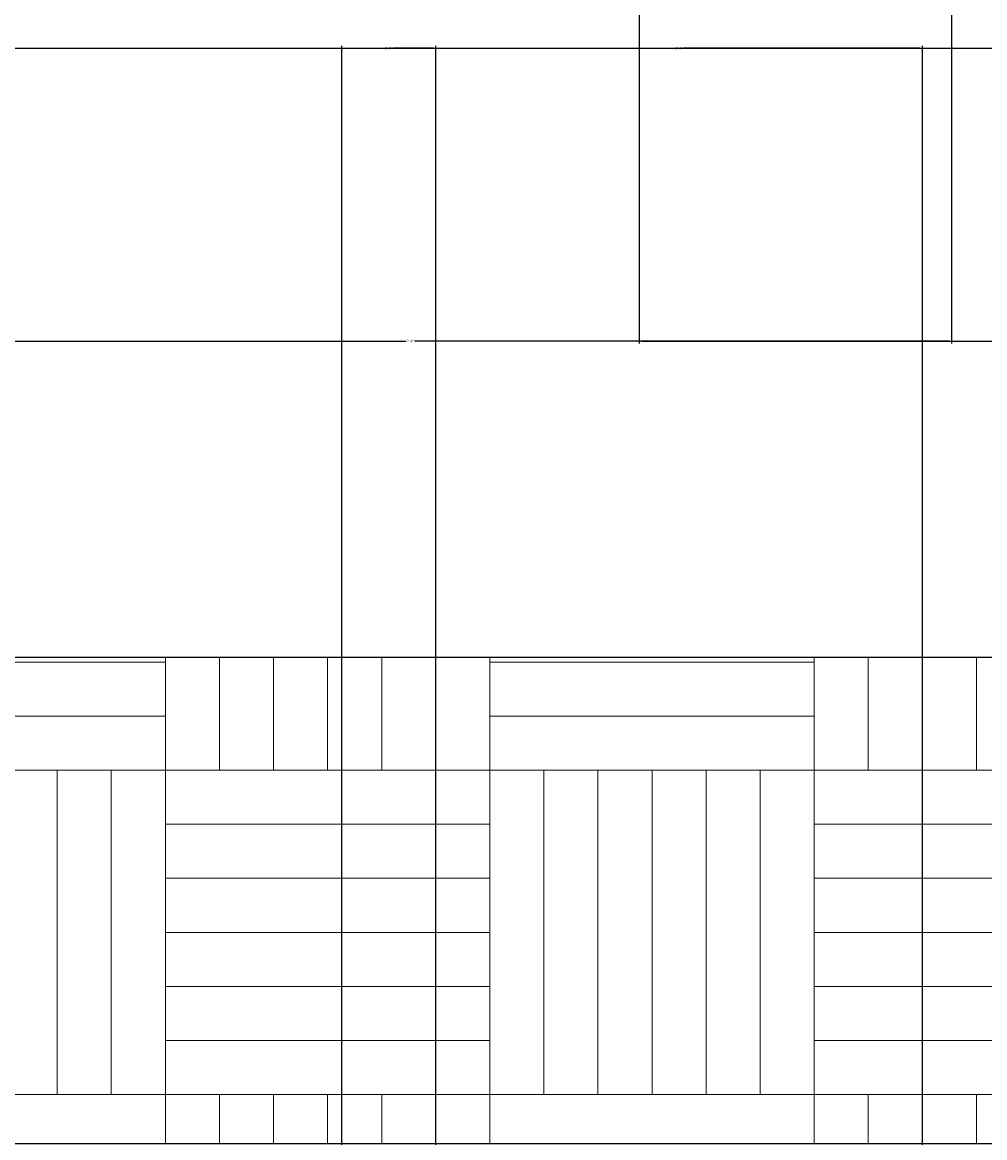
# Model space of a CAD drawing. Units: inches. Extents: x 37 to 824, y -700 to 234.
# Tile 8 of 77: x 181 to 253, y -459 to -377. Entities that reach past the tile are written whole.
import ezdxf

# ---------------------------------------------------------------- set-up
doc = ezdxf.new("R2010")
doc.units = ezdxf.units.IN
doc.header["$MEASUREMENT"] = 0
for name, color, linetype, lineweight in [('A-ANNO-DIMS', 2, 'Continuous', 18), ('A-ELEV', 3, 'Continuous', 25), ('A-ELEV-PATT', 8, 'Continuous', 13)]:
    doc.layers.add(name, color=color, linetype=linetype, lineweight=lineweight)
doc.styles.get("Standard").update_dxf_attribs({"font": 'arial.ttf'})
doc.dimstyles.get("Standard").update_dxf_attribs({"dimtxt": 0.18, "dimasz": 0.18, "dimexe": 0.18, "dimexo": 0.0625, "dimgap": 0.09, "dimtad": 0, "dimtih": 1, "dimtoh": 1, "dimdec": 1, "dimzin": 0, "dimdsep": 46, "dimlunit": 4, "dimtxsty": 'Standard', "dimcen": 0.09, "dimadec": 0, "dimazin": 0, "dimtfac": 1, "dimtdec": 1, "dimtofl": 0, "dimtmove": 0, "dimatfit": 3, "dimfxl": 1, "dimtolj": 1, "dimtzin": 0, "dimarcsym": 0})

# ---------------------------------------------------------------- blocks, each defined once
blk = doc.blocks.new('*D66')
at = {"layer": 'A-ANNO-DIMS', "color": 0, "lineweight": -2, "ltscale": 0.5, "transparency": 16777216}
for p, q in [((161.077, -423.565), (161.077, -378.38)), ((161.257, -378.56), (294.176, -378.56)), ((427.897, -378.56), (294.978, -378.56)), ((428.077, -423.565), (428.077, -378.38))]:
    blk.add_line(p, q, dxfattribs=at)
at = {"layer": 'A-ANNO-DIMS', "color": 0, "ltscale": 0.5, "transparency": 16777216}
for points in [[(161.257, -378.53), (161.257, -378.59), (161.077, -378.56)], [(427.897, -378.53), (427.897, -378.59), (428.077, -378.56)]]:
    blk.add_solid(points, dxfattribs=at)
at = {"layer": 'Defpoints', "color": 0, "ltscale": 0.5, "transparency": 16777216}
for p in [(428.077, -378.56), (161.077, -423.627), (428.077, -423.627)]:
    blk.add_point(p, dxfattribs=at)
at = {"layer": 'A-ANNO-DIMS', "color": 0, "ltscale": 0.5, "transparency": 16777216, "insert": (294.577, -378.56), "char_height": 0.18, "attachment_point": 5}
blk.add_mtext('\\A1;22\'-3"', dxfattribs=at)
blk = doc.blocks.new('*D77')
at = {"layer": 'A-ANNO-DIMS', "color": 0, "lineweight": -2, "ltscale": 0.5, "transparency": 16777216}
for p, q in [((227.077, 45.5), (227.077, -400.406)), ((290.077, 15.028), (290.077, -400.406)), ((227.257, -400.226), (258.248, -400.226)), ((289.897, -400.226), (258.906, -400.226))]:
    blk.add_line(p, q, dxfattribs=at)
at = {"layer": 'A-ANNO-DIMS', "color": 0, "ltscale": 0.5, "transparency": 16777216}
for points in [[(227.257, -400.196), (227.257, -400.256), (227.077, -400.226)], [(289.897, -400.196), (289.897, -400.256), (290.077, -400.226)]]:
    blk.add_solid(points, dxfattribs=at)
at = {"layer": 'Defpoints', "color": 0, "ltscale": 0.5, "transparency": 16777216}
for p in [(227.077, 45.563), (290.077, 15.09), (290.077, -400.226)]:
    blk.add_point(p, dxfattribs=at)
at = {"layer": 'A-ANNO-DIMS', "color": 0, "ltscale": 0.5, "transparency": 16777216, "insert": (258.577, -400.226), "char_height": 0.18, "attachment_point": 5}
blk.add_mtext('\\A1;5\'-3"', dxfattribs=at)
blk = doc.blocks.new('*D80')
at = {"layer": 'A-ANNO-DIMS', "color": 0, "lineweight": -2, "ltscale": 0.5, "transparency": 16777216}
for p, q in [((170.077, -167.972), (170.077, -400.406)), ((250.19, -167.972), (250.19, -400.406)), ((170.257, -400.226), (209.804, -400.226)), ((250.01, -400.226), (210.463, -400.226))]:
    blk.add_line(p, q, dxfattribs=at)
at = {"layer": 'A-ANNO-DIMS', "color": 0, "ltscale": 0.5, "transparency": 16777216}
for points in [[(170.257, -400.196), (170.257, -400.256), (170.077, -400.226)], [(250.01, -400.196), (250.01, -400.256), (250.19, -400.226)]]:
    blk.add_solid(points, dxfattribs=at)
at = {"layer": 'Defpoints', "color": 0, "ltscale": 0.5, "transparency": 16777216}
for p in [(170.077, -167.91), (250.19, -167.91), (250.19, -400.226)]:
    blk.add_point(p, dxfattribs=at)
at = {"layer": 'A-ANNO-DIMS', "color": 0, "ltscale": 0.5, "transparency": 16777216, "insert": (210.133, -400.226), "char_height": 0.18, "attachment_point": 5}
blk.add_mtext('\\A1;6\'-8"', dxfattribs=at)
blk = doc.blocks.new('*D81')
at = {"layer": 'A-ANNO-DIMS', "color": 0, "lineweight": -2, "ltscale": 0.5, "transparency": 16777216}
for p, q in [((290.077, -164.972), (290.077, -400.406)), ((250.19, -167.972), (250.19, -400.406)), ((250.37, -400.226), (269.804, -400.226)), ((289.897, -400.226), (270.463, -400.226))]:
    blk.add_line(p, q, dxfattribs=at)
at = {"layer": 'A-ANNO-DIMS', "color": 0, "ltscale": 0.5, "transparency": 16777216}
for points in [[(250.37, -400.196), (250.37, -400.256), (250.19, -400.226)], [(289.897, -400.196), (289.897, -400.256), (290.077, -400.226)]]:
    blk.add_solid(points, dxfattribs=at)
at = {"layer": 'Defpoints', "color": 0, "ltscale": 0.5, "transparency": 16777216}
for p in [(290.077, -164.91), (250.19, -167.91), (290.077, -400.226)]:
    blk.add_point(p, dxfattribs=at)
at = {"layer": 'A-ANNO-DIMS', "color": 0, "ltscale": 0.5, "transparency": 16777216, "insert": (270.133, -400.226), "char_height": 0.18, "attachment_point": 5}
blk.add_mtext('\\A1;3\'-4"', dxfattribs=at)
blk = doc.blocks.new('*D94')
at = {"layer": 'A-ANNO-DIMS', "color": 0, "lineweight": -2, "ltscale": 0.5, "transparency": 16777216}
for p, q in [((205.077, -489.565), (205.077, -378.38)), ((205.257, -378.56), (208.222, -378.56)), ((211.845, -378.56), (208.88, -378.56)), ((212.025, -495.652), (212.025, -378.38))]:
    blk.add_line(p, q, dxfattribs=at)
at = {"layer": 'A-ANNO-DIMS', "color": 0, "ltscale": 0.5, "transparency": 16777216}
for points in [[(205.257, -378.53), (205.257, -378.59), (205.077, -378.56)], [(211.845, -378.53), (211.845, -378.59), (212.025, -378.56)]]:
    blk.add_solid(points, dxfattribs=at)
at = {"layer": 'Defpoints', "color": 0, "ltscale": 0.5, "transparency": 16777216}
for p in [(212.025, -378.56), (205.077, -489.627), (212.025, -495.714)]:
    blk.add_point(p, dxfattribs=at)
at = {"layer": 'A-ANNO-DIMS', "color": 0, "ltscale": 0.5, "transparency": 16777216, "insert": (208.551, -378.56), "char_height": 0.18, "attachment_point": 5}
blk.add_mtext('\\A1;0\'-7"', dxfattribs=at)
blk = doc.blocks.new('*D95')
at = {"layer": 'A-ANNO-DIMS', "color": 0, "lineweight": -2, "ltscale": 0.5, "transparency": 16777216}
for p, q in [((212.025, -495.652), (212.025, -378.38)), ((212.205, -378.56), (229.696, -378.56)), ((247.845, -378.56), (230.354, -378.56)), ((248.025, -495.652), (248.025, -378.38))]:
    blk.add_line(p, q, dxfattribs=at)
at = {"layer": 'A-ANNO-DIMS', "color": 0, "ltscale": 0.5, "transparency": 16777216}
for points in [[(212.205, -378.53), (212.205, -378.59), (212.025, -378.56)], [(247.845, -378.53), (247.845, -378.59), (248.025, -378.56)]]:
    blk.add_solid(points, dxfattribs=at)
at = {"layer": 'Defpoints', "color": 0, "ltscale": 0.5, "transparency": 16777216}
for p in [(248.025, -378.56), (212.025, -495.714), (248.025, -495.714)]:
    blk.add_point(p, dxfattribs=at)
at = {"layer": 'A-ANNO-DIMS', "color": 0, "ltscale": 0.5, "transparency": 16777216, "insert": (230.025, -378.56), "char_height": 0.18, "attachment_point": 5}
blk.add_mtext('\\A1;3\'-0"', dxfattribs=at)

msp = doc.modelspace()

# ---------------------------------------------------------------- hatches: boundary and pattern name
at = {"layer": 'A-ELEV-PATT', "ltscale": 0.5}
h = msp.add_hatch(dxfattribs=at)
h.set_pattern_fill('AR-PARQ1', color=256, scale=2)
h.paths.add_polyline_path([(428.077, -423.627), (161.077, -423.627), (161.077, -459.627), (428.077, -459.627)])

# ---------------------------------------------------------------- linework, layer by layer
at = {"layer": 'A-ELEV', "ltscale": 0.5}
msp.add_lwpolyline([(161.077, -423.627), (428.077, -423.627), (428.077, -459.627), (161.077, -459.627)], close=True, dxfattribs=at)

# ---------------------------------------------------------------- dimensions: what is measured, and where the dimension line sits
at = {"layer": 'A-ANNO-DIMS', "ltscale": 0.5}
for base, p1, p2, picture, middle in [((290.077, -400.226), (227.077, 45.563), (290.077, 15.09), '*D77', (258.577, -400.226)), ((290.077, -400.226), (250.19, -167.91), (290.077, -164.91), '*D81', (270.133, -400.226)), ((250.19, -400.226), (170.077, -167.91), (250.19, -167.91), '*D80', (210.133, -400.226)), ((428.077, -378.56), (161.077, -423.627), (428.077, -423.627), '*D66', (294.577, -378.56)), ((212.025, -378.56), (205.077, -489.627), (212.025, -495.714), '*D94', (208.551, -378.56)), ((248.025, -378.56), (212.025, -495.714), (248.025, -495.714), '*D95', (230.025, -378.56))]:
    dim = msp.add_linear_dim(base=base, p1=p1, p2=p2, dimstyle='Standard', override={"dimdec": 1, "dimlfac": 1, "dimrnd": 0, "dimzin": 1, "dimdsep": 46, "dimlunit": 4, "dimfrac": 2}, dxfattribs=at)
    dim.commit()
    dim.dimension.update_dxf_attribs({"geometry": picture, "text_midpoint": middle})

doc.saveas('drawing.dxf')
